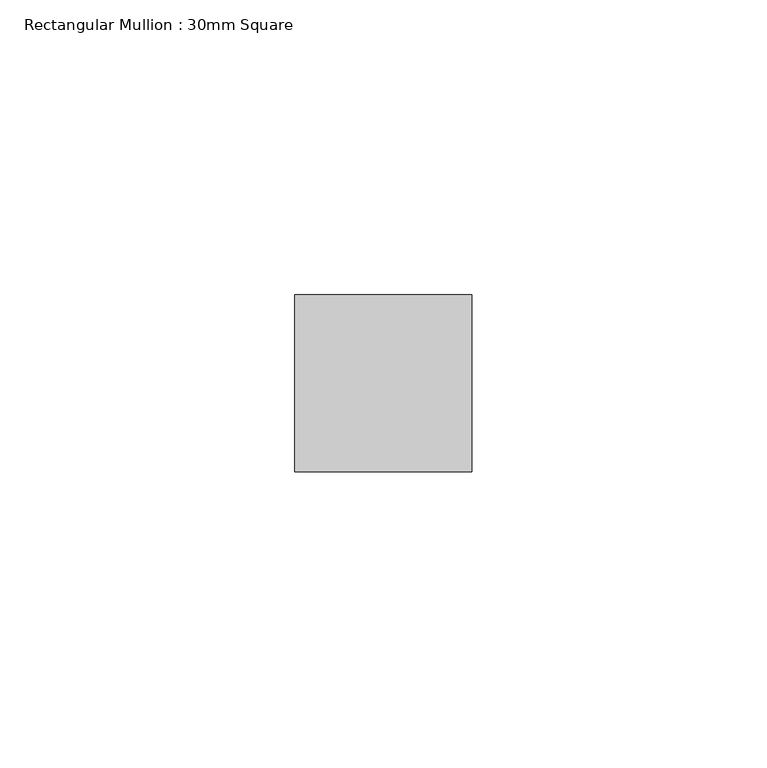
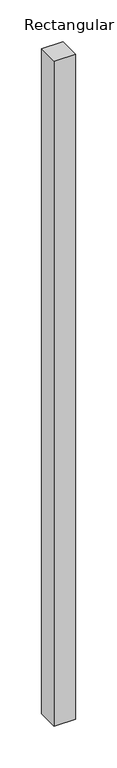
"""IFC4 building model written with IfcOpenShell, lengths in millimetres: member geometry, Rectangular Mullion : 30mm Square."""

from ifc_helpers import new_model, si_unit, frame, origin, place, context, project, spatial, polyline, outline, extrude, source, transform, mapped, element, save


def rectangular_mullion_30mm_square_038c5b05(model_context):
    return source(origin(), model_context, "Body", "SweptSolid", [
        extrude(outline(polyline([(15.0, 15.0), (15.0, -15.0), (-15.0, -15.0), (-15.0, 15.0), (15.0, 15.0)])), frame((0.0, 0.0, -975.0), z_axis=(0.0, 0.0, 1.0), x_axis=(1.0, 0.0, 0.0)), (0.0, 0.0, 1.0), 975.0),
    ])


if __name__ == "__main__":
    model = new_model("IFC4")
    model_context = context("Model", 3, world=origin())
    ifc_project = project(units=[si_unit("LENGTHUNIT", "METRE", prefix="MILLI")], contexts=[model_context])
    site = spatial("IfcSite", under=ifc_project)
    building = spatial("IfcBuilding", under=site)
    placement = place(None, origin())
    rectangular_mullion_30mm_square_shape = rectangular_mullion_30mm_square_038c5b05(model_context)
    element("IfcMember", 1, ObjectType="Rectangular Mullion : 30mm Square", at=placement, inside=building, context=model_context, shape_type="MappedRepresentation", body=[
        mapped(rectangular_mullion_30mm_square_shape, transform((0.0, 0.0, 0.0), x_axis=(1.0, 0.0, 0.0), y_axis=(0.0, 1.0, 0.0), z_axis=(0.0, 0.0, 1.0))),
    ])
    save(model, "model.ifc")

# Revit data of these elements
# Type "Rectangular Mullion : 30mm Square"
#   built-in parameter 1007304 = 0.0984252 (stored number, unit not read)
#   built-in parameter 1007301 = 0.0492126 (stored number, unit not read)
#   built-in parameter 1007300 = 0.0492126 (stored number, unit not read)
# Element 1 (IfcMember, "Rectangular Mullion : 30mm Square")
#   Materials on its faces: "Aluminum"
# Materials
#   "Aluminum": class "Metal", colour RGB 244 244 244, transparency 0, Description = "Aluminum 6061", Cost = 0
